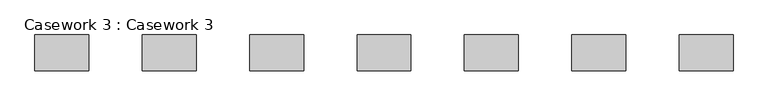
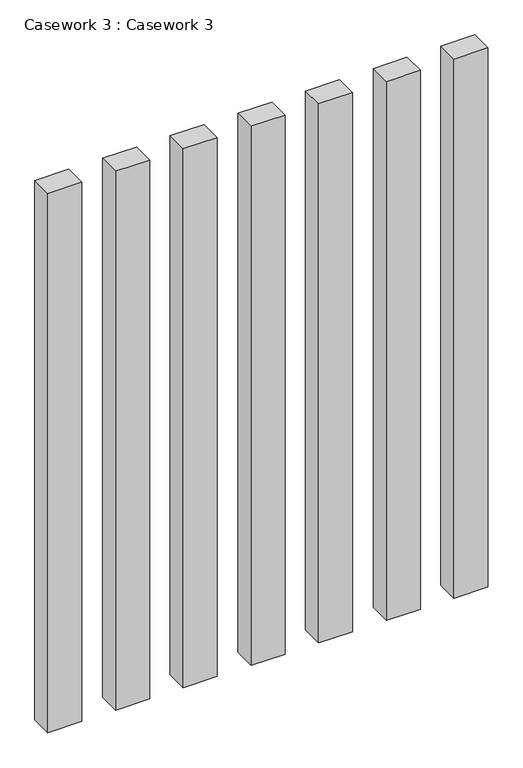
"""IFC4 building model written with IfcOpenShell, lengths in millimetres: furniture geometry, Casework 3 : Casework 3."""

from ifc_helpers import new_model, si_unit, frame, origin, place, context, project, spatial, polyline, outline, extrude, source, transform, mapped, element, save


def casework_3_casework_3_48862e2f(model_context):
    return source(origin(), model_context, "Body", "SweptSolid", [
        extrude(outline(polyline([(-16359.1792749, -1459.9833944), (-16509.1792749, -1459.9833944), (-16509.1792749, -1359.9833944), (-16359.1792749, -1359.9833944), (-16359.1792749, -1459.9833944)])), frame((0.0, 0.0, 3150.0), z_axis=(0.0, 0.0, 1.0), x_axis=(1.0, 0.0, 0.0)), (0.0, 0.0, 1.0), 2520.0),
        extrude(outline(polyline([(-16658.4790792, -1459.9833944), (-16808.4790792, -1459.9833944), (-16808.4790792, -1359.9833944), (-16658.4790792, -1359.9833944), (-16658.4790792, -1459.9833944)])), frame((0.0, 0.0, 3150.0), z_axis=(0.0, 0.0, 1.0), x_axis=(1.0, 0.0, 0.0)), (0.0, 0.0, 1.0), 2520.0),
        extrude(outline(polyline([(-16957.7788834, -1459.9833944), (-17107.7788834, -1459.9833944), (-17107.7788834, -1359.9833944), (-16957.7788834, -1359.9833944), (-16957.7788834, -1459.9833944)])), frame((0.0, 0.0, 3150.0), z_axis=(0.0, 0.0, 1.0), x_axis=(1.0, 0.0, 0.0)), (0.0, 0.0, 1.0), 2520.0),
        extrude(outline(polyline([(-17257.0786877, -1459.9833944), (-17407.0786877, -1459.9833944), (-17407.0786877, -1359.9833944), (-17257.0786877, -1359.9833944), (-17257.0786877, -1459.9833944)])), frame((0.0, 0.0, 3150.0), z_axis=(0.0, 0.0, 1.0), x_axis=(1.0, 0.0, 0.0)), (0.0, 0.0, 1.0), 2520.0),
        extrude(outline(polyline([(-17556.3784919, -1459.9833944), (-17706.3784919, -1459.9833944), (-17706.3784919, -1359.9833944), (-17556.3784919, -1359.9833944), (-17556.3784919, -1459.9833944)])), frame((0.0, 0.0, 3150.0), z_axis=(0.0, 0.0, 1.0), x_axis=(1.0, 0.0, 0.0)), (0.0, 0.0, 1.0), 2520.0),
        extrude(outline(polyline([(-17855.6782962, -1459.9833944), (-18005.6782962, -1459.9833944), (-18005.6782962, -1359.9833944), (-17855.6782962, -1359.9833944), (-17855.6782962, -1459.9833944)])), frame((0.0, 0.0, 3150.0), z_axis=(0.0, 0.0, 1.0), x_axis=(1.0, 0.0, 0.0)), (0.0, 0.0, 1.0), 2520.0),
        extrude(outline(polyline([(-18154.9781005, -1459.9833944), (-18304.9781005, -1459.9833944), (-18304.9781005, -1359.9833944), (-18154.9781005, -1359.9833944), (-18154.9781005, -1459.9833944)])), frame((0.0, 0.0, 3150.0), z_axis=(0.0, 0.0, 1.0), x_axis=(1.0, 0.0, 0.0)), (0.0, 0.0, 1.0), 2520.0),
    ])


if __name__ == "__main__":
    model = new_model("IFC4")
    model_context = context("Model", 3, world=origin())
    ifc_project = project(units=[si_unit("LENGTHUNIT", "METRE", prefix="MILLI")], contexts=[model_context])
    site = spatial("IfcSite", under=ifc_project)
    building = spatial("IfcBuilding", under=site)
    placement = place(None, origin())
    casework_3_casework_3_shape = casework_3_casework_3_48862e2f(model_context)
    element("IfcFurniture", 1, ObjectType="Casework 3 : Casework 3", at=placement, inside=building, context=model_context, shape_type="MappedRepresentation", body=[
        mapped(casework_3_casework_3_shape, transform((0.0, 0.0, 0.0), x_axis=(1.0, 0.0, 0.0), y_axis=(0.0, 1.0, 0.0), z_axis=(0.0, 0.0, 1.0))),
    ])
    save(model, "model.ifc")
